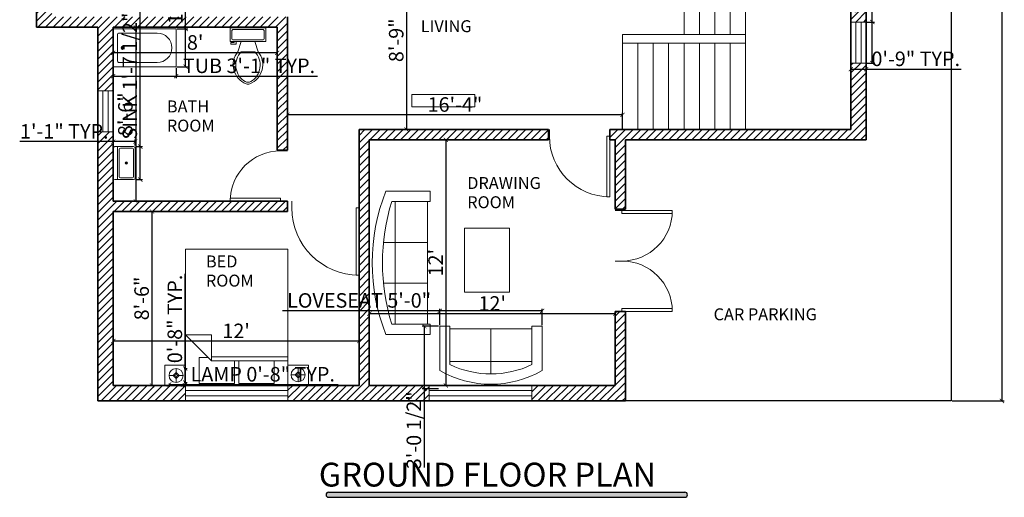
# Model space of a CAD drawing. Units: inches. Extents: x 3799 to 20199, y 1682 to 8087.
# Tile 18 of 30: x 14300 to 14876, y 2572 to 2852. Entities that reach past the tile are written whole.
import ezdxf

# ---------------------------------------------------------------- set-up
doc = ezdxf.new("R2010")
doc.units = ezdxf.units.IN
for name, color, linetype, lineweight in [('A-ANNO-DIMS', 2, 'Continuous', 18), ('A-ANNO-TITL', 7, 'Continuous', 25), ('A-AREA-IDEN', 7, 'Continuous', 18), ('A-DOOR', 3, 'Continuous', 18), ('A-FLOR-FIXT', 9, 'Continuous', 18), ('A-FLOR-STRS', 41, 'Continuous', 18), ('A-FURN', 8, 'Continuous', 18), ('A-GLAZ', 152, 'Continuous', 18), ('A-WALL', 7, 'Continuous', 35), ('A-WALL-PATT', 252, 'Continuous', 13), ('C-PROP', 7, 'Continuous', 25)]:
    doc.layers.add(name, color=color, linetype=linetype, lineweight=lineweight)
doc.styles.get("Standard").update_dxf_attribs({"font": 'arial.ttf'})
doc.dimstyles.new('ISO-25', dxfattribs={"dimtxt": 8.5, "dimasz": 2.5, "dimexe": 1.25, "dimexo": 0.625, "dimtad": 1, "dimdec": 0, "dimlunit": 3, "dimtxsty": 'Standard', "dimblk": 'ARCHTICK', "dimcen": 2.5, "dimadec": 0, "dimazin": 0, "dimtfac": 1, "dimtdec": 0, "dimtmove": 0, "dimatfit": 3, "dimfxl": 1, "dimarcsym": 0})

# ---------------------------------------------------------------- blocks, each defined once
blk = doc.blocks.new('Bed - Queen')
for p, q in [((0, -80.00003), (0, 0)), ((0, 0), (59.99999, 0)), ((59.99999, 0), (59.99999, -80.00003)), ((7.99999, -1.2), (28.79998, -1.2)), ((7.99999, -14.4), (7.99999, -1.2)), ((28.79998, -1.2), (28.79998, -14.4)), ((31.19999, -1.2), (51.99999, -1.2)), ((31.19999, -14.4), (31.19999, -1.2)), ((51.99999, -1.2), (51.99999, -16.4)), ((0, -14.4), (44.8, -14.4)), ((44.8, -16.8), (0, -16.8)), ((59.99999, -29.6), (44.8, -14.4)), ((44.8, -14.4), (44.8, -29.6)), ((51.99999, -16.4), (46.79936, -16.4)), ((44.8, -29.6), (59.99999, -29.6)), ((59.99999, -80.00003), (0, -80.00003))]:
    blk.add_line(p, q)
blk = doc.blocks.new('*U7')
for p, q in [((0, 0), (0, -100)), ((750, 0), (750, -100))]:
    blk.add_line(p, q)
blk.add_lwpolyline([(0, 0), (0, 750), (43.75, 750), (43.75, 0)], close=True)
blk.add_arc((0, 0), 750, 0, 90)
blk = doc.blocks.new('*U11')
for p, q in [((-900, 0), (-900, 100)), ((0, 0), (0, 100))]:
    blk.add_line(p, q)
blk.add_lwpolyline([(0, 0), (0, -900), (-43.75, -900), (-43.75, 0)], close=True)
blk.add_arc((0, 0), 900, 180, 270)
blk = doc.blocks.new('*U95')
for p, q in [((-1000, 0), (-1000, 100)), ((0, 0), (0, 100))]:
    blk.add_line(p, q)
blk.add_lwpolyline([(0, 0), (0, -1000), (-43.75, -1000), (-43.75, 0)], close=True)
blk.add_arc((0, 0), 1000, 180, 270)
blk = doc.blocks.new('Sofa - Roundback 7 ft.')
for p, q in [((-36.000027, -34), (-36.000027, -11.4696)), ((-12.00002, -32.4421), (-12.00003, -6.5971)), ((11.99997, -32.4421), (11.99998, -6.5971)), ((35.99998, -34), (35.99998, -11.4696)), ((-35.999844, -13.3819), (35.9998, -13.3819)), ((-36.000027, -32.4421), (35.99998, -32.4421))]:
    blk.add_line(p, q)
for points in [[(-36.000027, -34), (-42.000027, -34), (-42.000027, -8)], [(41.99998, -8), (41.99998, -34), (35.99998, -34)]]:
    blk.add_lwpolyline(points)
for centre, radius, start, end in [((0, -114.25), 114.25, 68.43141, 111.5686), ((-0.00001, -127.1968), 121.1968, 72.72033, 107.2797)]:
    blk.add_arc(centre, radius, start, end)
blk = doc.blocks.new('Sofa - Roundback Loveseat 5 ft.')
for p, q in [((-24, -33.99998), (-24, -11.46958)), ((0, -32.44198), (0, -5.99998)), ((24.00004, -33.99998), (24.00004, -11.46958)), ((-23.9998, -13.38178), (23.99986, -13.38178)), ((-24, -32.44198), (24.00004, -32.44198))]:
    blk.add_line(p, q)
for points in [[(-24, -33.99998), (-30, -33.99998), (-30, -7.99998)], [(30.00004, -7.99998), (30.00004, -33.99998), (24.00004, -33.99998)]]:
    blk.add_lwpolyline(points)
for centre, radius, start, end in [((0, -60.24998), 60.24998, 60.13715, 119.8628), ((0, -61.38438), 55.38444, 64.32083, 115.6792)]:
    blk.add_arc(centre, radius, start, end)
blk = doc.blocks.new('Lamp - Table')
for p, q in [((-1, 0), (-7, 0)), ((0, 3), (-3, 0)), ((-3, 0), (0, -3)), ((0, 7), (0, 1)), ((3, 0), (0, 3)), ((0, -3), (3, 0)), ((1, 0), (7, 0)), ((0, -1), (0, -7))]:
    blk.add_line(p, q)
for radius in [7, 1]:
    blk.add_circle((0, 0), radius)
blk = doc.blocks.new('Toilet - top')
for p, q in [((9.5, -6), (9.5, -2)), ((-10, -8.5), (-8, -8.5)), ((-10, -9.5), (-10, -8.5)), ((-7, -9.5), (-10, -9.5)), ((-8, -8.5), (-8, -8)), ((-7, -8), (-7, -9.5)), ((-4, -8), (-6, -14)), ((4, -8), (6, -14)), ((4, -14), (-4, -14))]:
    blk.add_line(p, q)
blk.add_lwpolyline([(10.5, -8), (10.5, 0), (-10.5, 0), (-10.5, -8)], close=True)
for points in [[(-9.5, -2), (-9.5, -6)], [(8.5, -1), (-8.5, -1)], [(-8.5, -7), (8.5, -7)]]:
    blk.add_lwpolyline(points)
for centre, radius, start, end in [((-8.62, -1.88), 0.884, 81.8699, 188.1301), ((8.62, -1.88), 0.884, 351.8699, 98.1301), ((-8.62, -6.12), 0.884, 171.8699, 278.1301), ((8.62, -6.12), 0.884, 261.8699, 8.1301), ((3.52, -21.58), 12.17, 141.46911, 247.97143), ((4.2, -21.82), 11.33, 136.36773, 238.94682), ((-3.52, -21.58), 12.17, 292.02843, 38.53071), ((-4.2, -21.82), 11.33, 301.05301, 43.63209), ((0, -27.88), 4, 245.73182, 294.26817), ((0, -29), 4, 254.86053, 285.13947)]:
    blk.add_arc(centre, radius, start, end)
blk = doc.blocks.new('Bath Tub - 26 x 60 in.')
for p, q in [((8, -18), (10, -18)), ((9, -17), (9, -19))]:
    blk.add_line(p, q)
blk.add_lwpolyline([(0, -36), (0, 0), (60, 0), (60, -36)], close=True)
for points in [[(4, -30), (4, -6)], [(6, -4), (42, -4)], [(42, -32), (6, -32)]]:
    blk.add_lwpolyline(points)
for radius in [1.5, 1]:
    blk.add_circle((9, -18), radius)
for centre, radius, start, end in [((5.75, -5.75), 1.77, 81.8699, 188.1301), ((42, -18), 14, 270, 90), ((5.75, -30.25), 1.77, 171.8699, 278.1301)]:
    blk.add_arc(centre, radius, start, end)
blk = doc.blocks.new('Sink-single - 30 in top')
blk.add_line((-15, -3.999996), (15, -3.999996))
for points in [[(-13.5, 0), (13.5, 0)], [(-15, -18.499996), (-15, -1.5)], [(-13.5, -17.499996), (-13.5, -6.499996)], [(-12.5, -5.499996), (12.5, -5.499996)], [(13.5, -6.499996), (13.5, -17.499996)], [(15, -1.5), (15, -18.499996)], [(13.5, -19.999996), (-13.5, -19.999996)], [(12.5, -18.499996), (-12.5, -18.499996)]]:
    blk.add_lwpolyline(points)
for radius in [1, 0.5]:
    blk.add_circle((0, -11.999996), radius)
for centre, radius, start, end in [((-13.5, -1.5), 1.5, 90, 180), ((-12.5, -6.499996), 1, 90, 180), ((12.5, -6.499996), 1, 0, 90), ((13.5, -1.5), 1.5, 0, 90), ((-12.5, -17.499996), 1, 180, 270), ((12.5, -17.499996), 1, 270, 0), ((-13.5, -18.499996), 1.5, 180, 270), ((13.5, -18.499996), 1.5, 270, 0)]:
    blk.add_arc(centre, radius, start, end)
blk = doc.blocks.new('_ArchTick')
at = {"color": 0, "linetype": 'ByBlock', "const_width": 0.15}
blk.add_lwpolyline([(-0.5, -0.5), (0.5, 0.5)], dxfattribs=at)
blk = doc.blocks.new('*D105')
at = {"layer": 'A-ANNO-DIMS', "color": 0, "lineweight": -2, "transparency": 16777216}
for p, q in [((14355.09, 2847.09), (14368.91, 2847.09)), ((14367.66, 2847.09), (14367.66, 2745.09)), ((14355.09, 2745.09), (14368.91, 2745.09))]:
    blk.add_line(p, q, dxfattribs=at)
at = {"layer": 'Defpoints', "color": 0, "transparency": 16777216}
for p in [(14354.46, 2847.09), (14354.46, 2745.09), (14367.66, 2745.09)]:
    blk.add_point(p, dxfattribs=at)
at = {"layer": 'A-ANNO-DIMS', "color": 0, "lineweight": -2, "transparency": 16777216, "xscale": 2.5, "yscale": 2.5, "zscale": 2.5}
for p, rotation in [((14367.66, 2847.09), 90), ((14367.66, 2745.09), 270)]:
    blk.add_blockref('_ArchTick', p, dxfattribs=dict(at, rotation=rotation))
at = {"layer": 'A-ANNO-DIMS', "color": 0, "transparency": 16777216, "insert": (14362.7, 2796.09), "char_height": 8.5, "attachment_point": 5, "rotation": 90}
blk.add_mtext('8\'-6"', dxfattribs=at)
blk = doc.blocks.new('*D106')
at = {"layer": 'A-ANNO-DIMS', "color": 0, "lineweight": -2, "transparency": 16777216}
for p, q in [((14354.46, 2846.47), (14354.46, 2830.85)), ((14450.46, 2846.47), (14450.46, 2830.85)), ((14450.46, 2832.1), (14354.46, 2832.1))]:
    blk.add_line(p, q, dxfattribs=at)
at = {"layer": 'Defpoints', "color": 0, "transparency": 16777216}
for p in [(14354.46, 2847.09), (14450.46, 2847.09), (14354.46, 2832.1)]:
    blk.add_point(p, dxfattribs=at)
at = {"layer": 'A-ANNO-DIMS', "color": 0, "lineweight": -2, "transparency": 16777216, "xscale": 2.5, "yscale": 2.5, "zscale": 2.5, "rotation": 180}
blk.add_blockref('_ArchTick', (14354.46, 2832.1), dxfattribs=at)
at = {"layer": 'A-ANNO-DIMS', "color": 0, "lineweight": -2, "transparency": 16777216, "xscale": 2.5, "yscale": 2.5, "zscale": 2.5}
blk.add_blockref('_ArchTick', (14450.46, 2832.1), dxfattribs=at)
at = {"layer": 'A-ANNO-DIMS', "color": 0, "transparency": 16777216, "insert": (14402.46, 2837.06), "char_height": 8.5, "attachment_point": 5}
blk.add_mtext("8'", dxfattribs=at)
blk = doc.blocks.new('*D107')
at = {"layer": 'A-ANNO-DIMS', "color": 0, "lineweight": -2, "transparency": 16777216}
for p, q in [((14354.46, 2637.72), (14354.46, 2664.35)), ((14498.46, 2637.72), (14498.46, 2664.35)), ((14498.46, 2663.1), (14354.46, 2663.1))]:
    blk.add_line(p, q, dxfattribs=at)
at = {"layer": 'Defpoints', "color": 0, "transparency": 16777216}
for p in [(14354.46, 2663.1), (14354.46, 2637.09), (14498.46, 2637.09)]:
    blk.add_point(p, dxfattribs=at)
at = {"layer": 'A-ANNO-DIMS', "color": 0, "lineweight": -2, "transparency": 16777216, "xscale": 2.5, "yscale": 2.5, "zscale": 2.5, "rotation": 180}
blk.add_blockref('_ArchTick', (14354.46, 2663.1), dxfattribs=at)
at = {"layer": 'A-ANNO-DIMS', "color": 0, "lineweight": -2, "transparency": 16777216, "xscale": 2.5, "yscale": 2.5, "zscale": 2.5}
blk.add_blockref('_ArchTick', (14498.46, 2663.1), dxfattribs=at)
at = {"layer": 'A-ANNO-DIMS', "color": 0, "transparency": 16777216, "insert": (14426.46, 2667.99), "char_height": 8.5, "attachment_point": 5}
blk.add_mtext("12'", dxfattribs=at)
blk = doc.blocks.new('*D108')
at = {"layer": 'A-ANNO-DIMS', "color": 0, "lineweight": -2, "transparency": 16777216}
for p, q in [((14355.09, 2739.09), (14378.43, 2739.09)), ((14377.18, 2739.09), (14377.18, 2637.09)), ((14355.09, 2637.09), (14378.43, 2637.09))]:
    blk.add_line(p, q, dxfattribs=at)
at = {"layer": 'Defpoints', "color": 0, "transparency": 16777216}
for p in [(14354.46, 2739.09), (14354.46, 2637.09), (14377.18, 2637.09)]:
    blk.add_point(p, dxfattribs=at)
at = {"layer": 'A-ANNO-DIMS', "color": 0, "lineweight": -2, "transparency": 16777216, "xscale": 2.5, "yscale": 2.5, "zscale": 2.5}
for p, rotation in [((14377.18, 2739.09), 90), ((14377.18, 2637.09), 270)]:
    blk.add_blockref('_ArchTick', p, dxfattribs=dict(at, rotation=rotation))
at = {"layer": 'A-ANNO-DIMS', "color": 0, "transparency": 16777216, "insert": (14372.21, 2688.09), "char_height": 8.5, "attachment_point": 5, "rotation": 90}
blk.add_mtext('8\'-6"', dxfattribs=at)
blk = doc.blocks.new('*D109')
at = {"layer": 'A-ANNO-DIMS', "color": 0, "lineweight": -2, "transparency": 16777216}
for p, q in [((14505.09, 2781.09), (14550.53, 2781.09)), ((14549.28, 2781.09), (14549.28, 2637.09)), ((14505.09, 2637.09), (14550.53, 2637.09))]:
    blk.add_line(p, q, dxfattribs=at)
at = {"layer": 'Defpoints', "color": 0, "transparency": 16777216}
for p in [(14504.46, 2781.09), (14504.46, 2637.09), (14549.28, 2637.09)]:
    blk.add_point(p, dxfattribs=at)
at = {"layer": 'A-ANNO-DIMS', "color": 0, "lineweight": -2, "transparency": 16777216, "xscale": 2.5, "yscale": 2.5, "zscale": 2.5}
for p, rotation in [((14549.28, 2781.09), 90), ((14549.28, 2637.09), 270)]:
    blk.add_blockref('_ArchTick', p, dxfattribs=dict(at, rotation=rotation))
at = {"layer": 'A-ANNO-DIMS', "color": 0, "transparency": 16777216, "insert": (14544.39, 2709.09), "char_height": 8.5, "attachment_point": 5, "rotation": 90}
blk.add_mtext("12'", dxfattribs=at)
blk = doc.blocks.new('*D110')
at = {"layer": 'A-ANNO-DIMS', "color": 0, "lineweight": -2, "transparency": 16777216}
for p, q in [((14504.46, 2637.72), (14504.46, 2680.43)), ((14648.46, 2679.18), (14504.46, 2679.18)), ((14648.46, 2637.72), (14648.46, 2680.43))]:
    blk.add_line(p, q, dxfattribs=at)
at = {"layer": 'Defpoints', "color": 0, "transparency": 16777216}
for p in [(14504.46, 2679.18), (14504.46, 2637.09), (14648.46, 2637.09)]:
    blk.add_point(p, dxfattribs=at)
at = {"layer": 'A-ANNO-DIMS', "color": 0, "lineweight": -2, "transparency": 16777216, "xscale": 2.5, "yscale": 2.5, "zscale": 2.5, "rotation": 180}
blk.add_blockref('_ArchTick', (14504.46, 2679.18), dxfattribs=at)
at = {"layer": 'A-ANNO-DIMS', "color": 0, "lineweight": -2, "transparency": 16777216, "xscale": 2.5, "yscale": 2.5, "zscale": 2.5}
blk.add_blockref('_ArchTick', (14648.46, 2679.18), dxfattribs=at)
at = {"layer": 'A-ANNO-DIMS', "color": 0, "transparency": 16777216, "insert": (14576.46, 2684.07), "char_height": 8.5, "attachment_point": 5}
blk.add_mtext("12'", dxfattribs=at)
blk = doc.blocks.new('*D111')
at = {"layer": 'A-ANNO-DIMS', "color": 0, "lineweight": -2, "transparency": 16777216}
for p, q in [((14456.46, 2787.72), (14456.46, 2796.97)), ((14652.78, 2787.72), (14652.78, 2796.97)), ((14652.78, 2795.72), (14456.46, 2795.72))]:
    blk.add_line(p, q, dxfattribs=at)
at = {"layer": 'Defpoints', "color": 0, "transparency": 16777216}
for p in [(14456.46, 2795.72), (14456.46, 2787.09), (14652.78, 2787.09)]:
    blk.add_point(p, dxfattribs=at)
at = {"layer": 'A-ANNO-DIMS', "color": 0, "lineweight": -2, "transparency": 16777216, "xscale": 2.5, "yscale": 2.5, "zscale": 2.5, "rotation": 180}
blk.add_blockref('_ArchTick', (14456.46, 2795.72), dxfattribs=at)
at = {"layer": 'A-ANNO-DIMS', "color": 0, "lineweight": -2, "transparency": 16777216, "xscale": 2.5, "yscale": 2.5, "zscale": 2.5}
blk.add_blockref('_ArchTick', (14652.78, 2795.72), dxfattribs=at)
at = {"layer": 'A-ANNO-DIMS', "color": 0, "transparency": 16777216, "insert": (14554.62, 2800.68), "char_height": 8.5, "attachment_point": 5}
blk.add_mtext('16\'-4"', dxfattribs=at)
blk = doc.blocks.new('*D112')
at = {"layer": 'A-ANNO-DIMS', "color": 0, "lineweight": -2, "transparency": 16777216}
for p, q in [((14538.58, 2891.79), (14525.03, 2891.79)), ((14526.28, 2891.79), (14526.28, 2787.09)), ((14538.58, 2787.09), (14525.03, 2787.09))]:
    blk.add_line(p, q, dxfattribs=at)
at = {"layer": 'Defpoints', "color": 0, "transparency": 16777216}
for p in [(14539.2, 2891.79), (14526.28, 2787.09), (14539.2, 2787.09)]:
    blk.add_point(p, dxfattribs=at)
at = {"layer": 'A-ANNO-DIMS', "color": 0, "lineweight": -2, "transparency": 16777216, "xscale": 2.5, "yscale": 2.5, "zscale": 2.5}
for p, rotation in [((14526.28, 2891.79), 90), ((14526.28, 2787.09), 270)]:
    blk.add_blockref('_ArchTick', p, dxfattribs=dict(at, rotation=rotation))
at = {"layer": 'A-ANNO-DIMS', "color": 0, "transparency": 16777216, "insert": (14521.32, 2839.44), "char_height": 8.5, "attachment_point": 5, "rotation": 90}
blk.add_mtext('8\'-9"', dxfattribs=at)
blk = doc.blocks.new('*D121')
at = {"layer": 'A-ANNO-DIMS', "color": 0, "lineweight": -2, "transparency": 16777216}
for p, q in [((14845.83, 3155.79), (14876.24, 3155.79)), ((14874.99, 3155.79), (14874.99, 2628.09)), ((14845.83, 2628.09), (14876.24, 2628.09))]:
    blk.add_line(p, q, dxfattribs=at)
at = {"layer": 'Defpoints', "color": 0, "transparency": 16777216}
for p in [(14845.2, 3155.79), (14845.2, 2628.09), (14874.99, 2628.09)]:
    blk.add_point(p, dxfattribs=at)
at = {"layer": 'A-ANNO-DIMS', "color": 0, "lineweight": -2, "transparency": 16777216, "xscale": 2.5, "yscale": 2.5, "zscale": 2.5}
for p, rotation in [((14874.99, 3155.79), 90), ((14874.99, 2628.09), 270)]:
    blk.add_blockref('_ArchTick', p, dxfattribs=dict(at, rotation=rotation))
at = {"layer": 'A-ANNO-DIMS', "color": 0, "transparency": 16777216, "insert": (14870.11, 2891.94), "char_height": 8.5, "attachment_point": 5, "rotation": 90}
blk.add_mtext("44'", dxfattribs=at)
blk = doc.blocks.new('WIN-24IN-9IN-FRAME')
for p, q in [((0, 24), (9, 24)), ((3, 0), (3, 24)), ((6, 0), (6, 24)), ((0, 0), (9, 0))]:
    blk.add_line(p, q)
blk = doc.blocks.new('WIN-60IN-9IN-FRAME')
for p, q in [((0, 9), (0, 0)), ((60, 6), (0, 6)), ((60, 9), (60, 0)), ((60, 3), (0, 3))]:
    blk.add_line(p, q)
blk = doc.blocks.new('*D242')
at = {"layer": 'A-ANNO-DIMS', "color": 0, "lineweight": -2, "transparency": 16777216}
for p, q in [((14799.06, 2850.1), (14799.06, 2961.41)), ((14796.09, 2850.1), (14800.31, 2850.1)), ((14799.06, 2826.1), (14799.06, 2850.1)), ((14796.09, 2826.1), (14800.31, 2826.1))]:
    blk.add_line(p, q, dxfattribs=at)
at = {"layer": 'Defpoints', "color": 0, "transparency": 16777216}
for p in [(14795.46, 2850.1), (14799.06, 2850.1), (14795.46, 2826.1)]:
    blk.add_point(p, dxfattribs=at)
at = {"layer": 'A-ANNO-DIMS', "color": 0, "lineweight": -2, "transparency": 16777216, "xscale": 2.5, "yscale": 2.5, "zscale": 2.5}
for p, rotation in [((14799.06, 2850.1), 90), ((14799.06, 2826.1), 270)]:
    blk.add_blockref('_ArchTick', p, dxfattribs=dict(at, rotation=rotation))
at = {"layer": 'A-ANNO-DIMS', "color": 0, "transparency": 16777216, "insert": (14794.04, 2907), "char_height": 8.5, "attachment_point": 5, "rotation": 90}
blk.add_mtext('WINDOW 2\'-0" TYP.', dxfattribs=at)
blk = doc.blocks.new('*D243')
at = {"layer": 'A-ANNO-DIMS', "color": 0, "lineweight": -2, "transparency": 16777216}
for p, q in [((14786.46, 2825.47), (14786.46, 2821.25)), ((14786.46, 2822.5), (14795.46, 2822.5)), ((14795.46, 2825.47), (14795.46, 2821.25)), ((14795.46, 2822.5), (14851.03, 2822.5))]:
    blk.add_line(p, q, dxfattribs=at)
at = {"layer": 'Defpoints', "color": 0, "transparency": 16777216}
for p in [(14786.46, 2826.1), (14795.46, 2826.1), (14795.46, 2822.5)]:
    blk.add_point(p, dxfattribs=at)
at = {"layer": 'A-ANNO-DIMS', "color": 0, "lineweight": -2, "transparency": 16777216, "xscale": 2.5, "yscale": 2.5, "zscale": 2.5, "rotation": 180}
blk.add_blockref('_ArchTick', (14786.46, 2822.5), dxfattribs=at)
at = {"layer": 'A-ANNO-DIMS', "color": 0, "lineweight": -2, "transparency": 16777216, "xscale": 2.5, "yscale": 2.5, "zscale": 2.5}
blk.add_blockref('_ArchTick', (14795.46, 2822.5), dxfattribs=at)
at = {"layer": 'A-ANNO-DIMS', "color": 0, "transparency": 16777216, "insert": (14824.5, 2827.46), "char_height": 8.5, "attachment_point": 5}
blk.add_mtext('0\'-9" TYP.', dxfattribs=at)
blk = doc.blocks.new('*D248')
at = {"layer": 'A-ANNO-DIMS', "color": 0, "lineweight": -2, "transparency": 16777216}
for p, q in [((14387.18, 2638.22), (14387.18, 2636.37)), ((14387.18, 2637.62), (14395.38, 2637.62)), ((14395.38, 2638.22), (14395.38, 2636.37)), ((14395.38, 2637.62), (14486.2, 2637.62))]:
    blk.add_line(p, q, dxfattribs=at)
at = {"layer": 'Defpoints', "color": 0, "transparency": 16777216}
for p in [(14387.18, 2638.85), (14395.38, 2638.85), (14395.38, 2637.62)]:
    blk.add_point(p, dxfattribs=at)
at = {"layer": 'A-ANNO-DIMS', "color": 0, "lineweight": -2, "transparency": 16777216, "xscale": 2.5, "yscale": 2.5, "zscale": 2.5, "rotation": 180}
blk.add_blockref('_ArchTick', (14387.18, 2637.62), dxfattribs=at)
at = {"layer": 'A-ANNO-DIMS', "color": 0, "lineweight": -2, "transparency": 16777216, "xscale": 2.5, "yscale": 2.5, "zscale": 2.5}
blk.add_blockref('_ArchTick', (14395.38, 2637.62), dxfattribs=at)
at = {"layer": 'A-ANNO-DIMS', "color": 0, "transparency": 16777216, "insert": (14442.04, 2642.58), "char_height": 8.5, "attachment_point": 5}
blk.add_mtext('LAMP 0\'-8" TYP.', dxfattribs=at)
blk = doc.blocks.new('*D249')
at = {"layer": 'A-ANNO-DIMS', "color": 0, "lineweight": -2, "transparency": 16777216}
for p, q in [((14396.62, 2647.05), (14396.62, 2702.62)), ((14396.01, 2647.05), (14397.87, 2647.05)), ((14396.62, 2638.85), (14396.62, 2647.05)), ((14396.01, 2638.85), (14397.87, 2638.85))]:
    blk.add_line(p, q, dxfattribs=at)
at = {"layer": 'Defpoints', "color": 0, "transparency": 16777216}
for p in [(14395.38, 2647.05), (14396.62, 2647.05), (14395.38, 2638.85)]:
    blk.add_point(p, dxfattribs=at)
at = {"layer": 'A-ANNO-DIMS', "color": 0, "lineweight": -2, "transparency": 16777216, "xscale": 2.5, "yscale": 2.5, "zscale": 2.5}
for p, rotation in [((14396.62, 2647.05), 90), ((14396.62, 2638.85), 270)]:
    blk.add_blockref('_ArchTick', p, dxfattribs=dict(at, rotation=rotation))
at = {"layer": 'A-ANNO-DIMS', "color": 0, "transparency": 16777216, "insert": (14391.65, 2676.09), "char_height": 8.5, "attachment_point": 5, "rotation": 90}
blk.add_mtext('0\'-8" TYP.', dxfattribs=at)
blk = doc.blocks.new('*D276')
at = {"layer": 'A-ANNO-DIMS', "color": 0, "lineweight": -2, "transparency": 16777216}
for p, q in [((14545.69, 2672.47), (14545.69, 2682.09)), ((14605.69, 2672.47), (14605.69, 2682.09)), ((14545.69, 2680.84), (14453.72, 2680.84)), ((14605.69, 2680.84), (14545.69, 2680.84))]:
    blk.add_line(p, q, dxfattribs=at)
at = {"layer": 'Defpoints', "color": 0, "transparency": 16777216}
for p in [(14545.69, 2680.84), (14545.69, 2671.84), (14605.69, 2671.84)]:
    blk.add_point(p, dxfattribs=at)
at = {"layer": 'A-ANNO-DIMS', "color": 0, "lineweight": -2, "transparency": 16777216, "xscale": 2.5, "yscale": 2.5, "zscale": 2.5, "rotation": 180}
blk.add_blockref('_ArchTick', (14545.69, 2680.84), dxfattribs=at)
at = {"layer": 'A-ANNO-DIMS', "color": 0, "lineweight": -2, "transparency": 16777216, "xscale": 2.5, "yscale": 2.5, "zscale": 2.5}
blk.add_blockref('_ArchTick', (14605.69, 2680.84), dxfattribs=at)
at = {"layer": 'A-ANNO-DIMS', "color": 0, "transparency": 16777216, "insert": (14498.46, 2685.86), "char_height": 8.5, "attachment_point": 5}
blk.add_mtext('LOVESEAT 5\'-0"', dxfattribs=at)
blk = doc.blocks.new('*D277')
at = {"layer": 'A-ANNO-DIMS', "color": 0, "lineweight": -2, "transparency": 16777216}
for p, q in [((14545.06, 2671.84), (14535.44, 2671.84)), ((14536.69, 2671.84), (14536.69, 2635.18)), ((14545.06, 2635.18), (14535.44, 2635.18)), ((14536.69, 2635.18), (14536.69, 2589.03))]:
    blk.add_line(p, q, dxfattribs=at)
at = {"layer": 'Defpoints', "color": 0, "transparency": 16777216}
for p in [(14545.69, 2671.84), (14536.69, 2635.18), (14545.69, 2635.18)]:
    blk.add_point(p, dxfattribs=at)
at = {"layer": 'A-ANNO-DIMS', "color": 0, "lineweight": -2, "transparency": 16777216, "xscale": 2.5, "yscale": 2.5, "zscale": 2.5}
for p, rotation in [((14536.69, 2671.84), 90), ((14536.69, 2635.18), 270)]:
    blk.add_blockref('_ArchTick', p, dxfattribs=dict(at, rotation=rotation))
at = {"layer": 'A-ANNO-DIMS', "color": 0, "transparency": 16777216, "insert": (14531.66, 2610.85), "char_height": 8.5, "attachment_point": 5, "rotation": 90}
blk.add_mtext('3\'-0 1/2"', dxfattribs=at)
blk = doc.blocks.new('*D304')
at = {"layer": 'A-ANNO-DIMS', "color": 0, "lineweight": -2, "transparency": 16777216}
for p, q in [((14354.46, 2823.32), (14354.46, 2817.17)), ((14391.34, 2823.32), (14391.34, 2817.17)), ((14354.46, 2818.42), (14391.34, 2818.42)), ((14391.34, 2818.42), (14474.17, 2818.42))]:
    blk.add_line(p, q, dxfattribs=at)
at = {"layer": 'Defpoints', "color": 0, "transparency": 16777216}
for p in [(14354.46, 2823.95), (14391.34, 2823.95), (14391.34, 2818.42)]:
    blk.add_point(p, dxfattribs=at)
at = {"layer": 'A-ANNO-DIMS', "color": 0, "lineweight": -2, "transparency": 16777216, "xscale": 2.5, "yscale": 2.5, "zscale": 2.5, "rotation": 180}
blk.add_blockref('_ArchTick', (14354.46, 2818.42), dxfattribs=at)
at = {"layer": 'A-ANNO-DIMS', "color": 0, "lineweight": -2, "transparency": 16777216, "xscale": 2.5, "yscale": 2.5, "zscale": 2.5}
blk.add_blockref('_ArchTick', (14391.34, 2818.42), dxfattribs=at)
at = {"layer": 'A-ANNO-DIMS', "color": 0, "transparency": 16777216, "insert": (14434, 2823.38), "char_height": 8.5, "attachment_point": 5}
blk.add_mtext('TUB 3\'-1" TYP.', dxfattribs=at)
blk = doc.blocks.new('*D305')
at = {"layer": 'A-ANNO-DIMS', "color": 0, "lineweight": -2, "transparency": 16777216}
for p, q in [((14396.87, 2846.08), (14396.87, 2907.44)), ((14391.97, 2846.08), (14398.12, 2846.08)), ((14396.87, 2823.95), (14396.87, 2846.08)), ((14391.97, 2823.95), (14398.12, 2823.95))]:
    blk.add_line(p, q, dxfattribs=at)
at = {"layer": 'Defpoints', "color": 0, "transparency": 16777216}
for p in [(14391.34, 2846.08), (14396.87, 2846.08), (14391.34, 2823.95)]:
    blk.add_point(p, dxfattribs=at)
at = {"layer": 'A-ANNO-DIMS', "color": 0, "lineweight": -2, "transparency": 16777216, "xscale": 2.5, "yscale": 2.5, "zscale": 2.5}
for p, rotation in [((14396.87, 2846.08), 90), ((14396.87, 2823.95), 270)]:
    blk.add_blockref('_ArchTick', p, dxfattribs=dict(at, rotation=rotation))
at = {"layer": 'A-ANNO-DIMS', "color": 0, "transparency": 16777216, "insert": (14391.91, 2878.01), "char_height": 8.5, "attachment_point": 5, "rotation": 90}
blk.add_mtext('1\'-10" TYP.', dxfattribs=at)
blk = doc.blocks.new('*D320')
at = {"layer": 'A-ANNO-DIMS', "color": 0, "lineweight": -2, "transparency": 16777216}
for p, q in [((14370.29, 2777.14), (14370.29, 2883.48)), ((14368.01, 2777.14), (14371.54, 2777.14)), ((14370.29, 2757.76), (14370.29, 2777.14)), ((14368.01, 2757.76), (14371.54, 2757.76))]:
    blk.add_line(p, q, dxfattribs=at)
at = {"layer": 'Defpoints', "color": 0, "transparency": 16777216}
for p in [(14367.39, 2777.14), (14370.29, 2777.14), (14367.39, 2757.76)]:
    blk.add_point(p, dxfattribs=at)
at = {"layer": 'A-ANNO-DIMS', "color": 0, "lineweight": -2, "transparency": 16777216, "xscale": 2.5, "yscale": 2.5, "zscale": 2.5}
for p, rotation in [((14370.29, 2777.14), 90), ((14370.29, 2757.76), 270)]:
    blk.add_blockref('_ArchTick', p, dxfattribs=dict(at, rotation=rotation))
at = {"layer": 'A-ANNO-DIMS', "color": 0, "transparency": 16777216, "insert": (14365.27, 2831.56), "char_height": 8.5, "attachment_point": 5, "rotation": 90}
blk.add_mtext('SINK 1\'-7 1/2" TYP.', dxfattribs=at)
blk = doc.blocks.new('*D321')
at = {"layer": 'A-ANNO-DIMS', "color": 0, "lineweight": -2, "transparency": 16777216}
for p, q in [((14354.46, 2780.04), (14299.7, 2780.04)), ((14354.46, 2777.76), (14354.46, 2781.29)), ((14367.39, 2780.04), (14354.46, 2780.04)), ((14367.39, 2777.76), (14367.39, 2781.29))]:
    blk.add_line(p, q, dxfattribs=at)
at = {"layer": 'Defpoints', "color": 0, "transparency": 16777216}
for p in [(14354.46, 2780.04), (14354.46, 2777.14), (14367.39, 2777.14)]:
    blk.add_point(p, dxfattribs=at)
at = {"layer": 'A-ANNO-DIMS', "color": 0, "lineweight": -2, "transparency": 16777216, "xscale": 2.5, "yscale": 2.5, "zscale": 2.5, "rotation": 180}
blk.add_blockref('_ArchTick', (14354.46, 2780.04), dxfattribs=at)
at = {"layer": 'A-ANNO-DIMS', "color": 0, "lineweight": -2, "transparency": 16777216, "xscale": 2.5, "yscale": 2.5, "zscale": 2.5}
blk.add_blockref('_ArchTick', (14367.39, 2780.04), dxfattribs=at)
at = {"layer": 'A-ANNO-DIMS', "color": 0, "transparency": 16777216, "insert": (14325.83, 2784.94), "char_height": 8.5, "attachment_point": 5}
blk.add_mtext('1\'-1" TYP.', dxfattribs=at)

msp = doc.modelspace()

# ---------------------------------------------------------------- hatches: boundary and pattern name
at = {"layer": 'A-ANNO-TITL'}
h = msp.add_hatch(color=256, dxfattribs=at)
h.dxf.hatch_style = 1
h.paths.add_polyline_path([(14689.33, 2574.54), (14480.6, 2574.54, 1), (14480.6, 2571.54), (14689.33, 2571.54, 1)])
at = {"layer": 'A-WALL-PATT'}
h = msp.add_hatch(dxfattribs=at)
h.set_pattern_fill('ANSI31', color=256)
h.paths.add_polyline_path([(14318.46, 2965.3), (14318.46, 2981.76), (14420.46, 2981.76), (14420.46, 2987.76), (14318.46, 2987.76), (14318.46, 3083.76), (14369.36, 3083.76), (14369.36, 3092.76), (14309.46, 3092.76), (14309.46, 2953.3), (14318.46, 2953.3)])
h.paths.add_polyline_path([(14456.46, 3092.76), (14393.36, 3092.76), (14393.36, 3083.76), (14450.46, 3083.76), (14450.46, 2987.76), (14450.46, 2981.76), (14450.46, 2889.09), (14456.46, 2889.09), (14456.46, 2891.79), (14539.2, 2891.79), (14539.2, 2945.79), (14533.2, 2945.79), (14533.2, 2897.79), (14456.46, 2897.79), (14456.46, 3065.79), (14474.23, 3065.79), (14474.23, 3074.79), (14456.46, 3074.79)])
h.paths.add_polyline_path([(14480.23, 3119.94, -0.534305), (14576.23, 3119.94), (14576.23, 3065.79), (14582.23, 3065.79), (14582.23, 3119.79, 0.570302), (14474.23, 3119.79), (14474.23, 3065.79), (14480.23, 3065.79)])
h.paths.add_polyline_path([(14608.2, 3146.79), (14728.2, 3146.79), (14728.2, 3109.9), (14737.2, 3109.9), (14737.2, 3155.79), (14599.2, 3155.79), (14599.2, 3074.79), (14582.23, 3074.79), (14582.23, 3065.79), (14602.2, 3065.79), (14602.2, 2936.79), (14608.2, 2936.79)])
h.paths.add_polyline_path([(14737.2, 3085.9), (14728.2, 3085.9), (14728.2, 3074.79), (14638.2, 3074.79), (14638.2, 3068.79), (14728.2, 3068.79), (14728.2, 3053.38), (14737.2, 3053.38)], flags=17)
h.paths.add_polyline_path([(14737.2, 2993.38), (14728.2, 2993.38), (14728.2, 2900.79), (14599.2, 2900.79), (14599.2, 2894.79), (14737.2, 2894.79)])
h.paths.add_polyline_path([(14795.46, 2897.45), (14791.43, 2897.45), (14791.43, 2897.79), (14772.64, 2897.79), (14772.64, 2894.79), (14786.46, 2894.79), (14786.46, 2850.1), (14795.46, 2850.1)])
h.paths.add_polyline_path([(14795.46, 2826.1), (14786.46, 2826.1), (14786.46, 2787.09), (14645.38, 2787.09), (14645.38, 2781.09), (14648.46, 2781.09), (14648.46, 2740.52), (14654.46, 2740.52), (14654.46, 2781.09), (14795.46, 2781.09)])
h.paths.add_polyline_path([(14654.46, 2680.52), (14648.46, 2680.52), (14648.46, 2637.09), (14599.58, 2637.09), (14599.58, 2628.09), (14654.46, 2628.09)])
h.paths.add_polyline_path([(14539.58, 2637.09), (14504.46, 2637.09), (14504.46, 2781.09), (14609.38, 2781.09), (14609.38, 2787.09), (14498.46, 2787.09), (14498.46, 2637.09), (14456.79, 2637.09), (14456.79, 2628.09), (14539.58, 2628.09)])
h.paths.add_polyline_path([(14396.79, 2637.09), (14384.79, 2637.09), (14354.46, 2637.09), (14354.46, 2739.09), (14456.46, 2739.09), (14456.46, 2745.09), (14354.46, 2745.09), (14354.46, 2785.72), (14345.46, 2785.72), (14345.46, 2628.09), (14396.79, 2628.09)])
h.paths.add_polyline_path([(14456.46, 2853.09), (14450.46, 2853.09), (14318.46, 2853.09), (14318.46, 2893.3), (14309.46, 2893.3), (14309.46, 2847.09), (14345.46, 2847.09), (14345.46, 2809.72), (14354.46, 2809.72), (14354.46, 2847.09), (14450.46, 2847.09), (14450.46, 2775.09), (14456.46, 2775.09)])

# ---------------------------------------------------------------- linework, layer by layer
at = {"layer": 'A-ANNO-TITL'}
for p, q in [((14480.6, 2574.54), (14689.33, 2574.54)), ((14480.6, 2571.54), (14689.33, 2571.54))]:
    msp.add_line(p, q, dxfattribs=at)
for centre, start, end in [((14480.6, 2573.04), 90, 270), ((14689.33, 2573.04), 270, 90)]:
    msp.add_arc(centre, 1.5, start, end, dxfattribs=at)
at = {"layer": 'A-FLOR-STRS'}
for p, q in [((14688.78, 2894.79), (14688.78, 2842.79)), ((14697.78, 2894.79), (14697.78, 2842.79)), ((14706.78, 2894.79), (14706.78, 2842.79)), ((14715.78, 2894.79), (14715.78, 2842.79)), ((14724.78, 2894.79), (14724.78, 2787.09)), ((14652.78, 2842.79), (14652.78, 2787.09)), ((14724.78, 2842.79), (14652.78, 2842.79)), ((14724.78, 2837.79), (14652.78, 2837.79)), ((14661.78, 2837.79), (14661.78, 2787.09)), ((14670.78, 2837.79), (14670.78, 2787.09)), ((14670.78, 2837.79), (14670.78, 2787.09)), ((14679.78, 2837.79), (14679.78, 2787.09)), ((14688.78, 2837.79), (14688.78, 2787.09)), ((14697.78, 2837.79), (14697.78, 2787.09)), ((14706.78, 2837.79), (14706.78, 2787.09)), ((14715.78, 2837.79), (14715.78, 2787.09))]:
    msp.add_line(p, q, dxfattribs=at)
at = {"layer": 'A-FURN'}
for points in [[(14529.37, 2807.66), (14566.27, 2807.66), (14566.27, 2800.34), (14529.37, 2800.34)], [(14560.19, 2729.23), (14586.57, 2729.23), (14586.57, 2691.88), (14560.19, 2691.88)], [(14396.79, 2637.09), (14384.79, 2637.09), (14384.79, 2649.09), (14396.79, 2649.09)], [(14456.79, 2637.09), (14468.79, 2637.09), (14468.79, 2649.09), (14456.79, 2649.09)]]:
    msp.add_lwpolyline(points, close=True, dxfattribs=at)
at = {"layer": 'A-WALL'}
for p, q in [((14309.46, 3092.76), (14309.46, 2847.09)), ((14795.46, 2781.09), (14795.46, 2897.45)), ((14786.46, 2787.09), (14786.46, 2894.79)), ((14456.46, 2853.09), (14456.46, 2775.09)), ((14345.46, 2847.09), (14309.46, 2847.09)), ((14345.46, 2847.09), (14345.46, 2628.09)), ((14450.46, 2847.09), (14354.46, 2847.09)), ((14354.46, 2847.09), (14354.46, 2745.09)), ((14450.46, 2847.09), (14450.46, 2775.09)), ((14498.46, 2787.09), (14498.46, 2637.09)), ((14609.38, 2787.09), (14498.46, 2787.09)), ((14609.38, 2781.09), (14609.38, 2787.09)), ((14786.46, 2787.09), (14645.38, 2787.09)), ((14645.38, 2781.09), (14645.38, 2787.09)), ((14504.46, 2781.09), (14504.46, 2637.09)), ((14609.38, 2781.09), (14504.46, 2781.09)), ((14648.46, 2781.09), (14645.38, 2781.09)), ((14648.46, 2781.09), (14648.46, 2740.52)), ((14795.46, 2781.09), (14654.46, 2781.09)), ((14654.46, 2781.09), (14654.46, 2740.52)), ((14456.46, 2775.09), (14450.46, 2775.09)), ((14456.46, 2745.09), (14354.46, 2745.09)), ((14456.46, 2745.09), (14456.46, 2739.09)), ((14648.46, 2740.52), (14654.46, 2740.52)), ((14456.46, 2739.09), (14354.46, 2739.09)), ((14354.46, 2739.09), (14354.46, 2637.09)), ((14648.46, 2680.52), (14654.46, 2680.52)), ((14648.46, 2680.52), (14648.46, 2637.09)), ((14654.46, 2680.52), (14654.46, 2628.09)), ((14498.46, 2637.09), (14354.46, 2637.09)), ((14648.46, 2637.09), (14504.46, 2637.09)), ((14654.46, 2628.09), (14345.46, 2628.09))]:
    msp.add_line(p, q, dxfattribs=at)
at = {"layer": 'C-PROP'}
for p, q in [((14845.2, 3155.79), (14845.2, 2628.09)), ((14845.2, 2628.09), (14654.46, 2628.09))]:
    msp.add_line(p, q, dxfattribs=at)

# ---------------------------------------------------------------- block references
at = {"layer": 'A-DOOR', "xscale": 0.0393700787401575, "yscale": 0.0393700787401575, "zscale": 0.0393700787401575}
for name, p in [('*U11', (14645.38, 2783.15)), ('*U95', (14498.46, 2741.15))]:
    msp.add_blockref(name, p, dxfattribs=at)
at = {"layer": 'A-DOOR', "yscale": 0.0393700787401575, "zscale": 0.0393700787401575}
for p, xscale, rotation in [((14452.53, 2745.09), 0.0393700787401575, 90), ((14652.4, 2739.58), 0.0393700787401575, 270), ((14652.4, 2680.52), -0.0393700787401575, 270)]:
    msp.add_blockref('*U7', p, dxfattribs=dict(at, xscale=xscale, rotation=rotation))
at = {"layer": 'A-FLOR-FIXT', "xscale": 0.6146362971528592, "yscale": 0.6146362971528592, "zscale": 0.6146362971528592}
msp.add_blockref('Bath Tub - 26 x 60 in.', (14354.46, 2846.08), dxfattribs=at)
at = {"layer": 'A-FLOR-FIXT'}
msp.add_blockref('Toilet - top', (14433.41, 2846.71), dxfattribs=at)
at = {"layer": 'A-FLOR-FIXT', "xscale": 0.6460358096658105, "yscale": 0.6460358096658105, "zscale": 0.6460358096658105, "rotation": 90}
msp.add_blockref('Sink-single - 30 in top', (14354.46, 2767.45), dxfattribs=at)
at = {"layer": 'A-FURN'}
for name, p, rotation in [('Sofa - Roundback 7 ft.', (14506.18, 2708.99), 90), ('Bed - Queen', (14456.79, 2637.09), 180), ('Sofa - Roundback Loveseat 5 ft.', (14575.69, 2637.84), 180)]:
    msp.add_blockref(name, p, dxfattribs=dict(at, rotation=rotation))
at = {"layer": 'A-FURN', "xscale": 0.5860159880705021, "yscale": 0.5860159880705021, "zscale": 0.5860159880705021}
for p in [(14391.28, 2642.95), (14462.74, 2643.37)]:
    msp.add_blockref('Lamp - Table', p, dxfattribs=at)
at = {"layer": 'A-GLAZ'}
for name, p in [('WIN-24IN-9IN-FRAME', (14786.46, 2826.1)), ('WIN-24IN-9IN-FRAME', (14345.46, 2785.72)), ('WIN-60IN-9IN-FRAME', (14396.79, 2628.09)), ('WIN-60IN-9IN-FRAME', (14539.58, 2628.09))]:
    msp.add_blockref(name, p, dxfattribs=at)

# ---------------------------------------------------------------- texts
at = {"layer": 'A-ANNO-TITL'}
msp.add_text('GROUND FLOOR PLAN', height=13.966, rotation=0.00194, dxfattribs=at).set_placement((14474.89, 2577.86))
at = {"layer": 'A-AREA-IDEN'}
for s, p in [('LIVING', (14534.6, 2844.19)), ('BATH', (14385.9, 2797.16)), ('ROOM', (14385.9, 2785.92)), ('DRAWING', (14561.81, 2752.26)), ('ROOM', (14561.81, 2741.01)), ('BED', (14408.77, 2706.3)), ('ROOM', (14408.77, 2695.06)), ('CAR PARKING', (14706.11, 2675.31))]:
    msp.add_text(s, height=7, rotation=0.00194, dxfattribs=at).set_placement(p)

# ---------------------------------------------------------------- dimensions: what is measured, and where the dimension line sits
at = {"layer": 'A-ANNO-DIMS'}
for base, p1, p2, angle, override, picture, middle in [((14874.99, 2628.09), (14845.2, 3155.79), (14845.2, 2628.09), 90, {"dimclrd": 0, "dimclre": 0, "dimclrt": 0}, '*D121', (14870.11, 2891.94)), ((14526.28, 2787.09), (14539.2, 2891.79), (14539.2, 2787.09), 90, {"dimclrd": 0, "dimclre": 0, "dimclrt": 0}, '*D112', (14521.32, 2839.44)), ((14377.18, 2637.09), (14354.46, 2739.09), (14354.46, 2637.09), 90, {"dimclrd": 0, "dimclre": 0, "dimclrt": 0}, '*D108', (14372.21, 2688.09)), ((14536.69, 2635.18), (14545.69, 2671.84), (14545.69, 2635.18), 270, {"dimdec": 1, "dimlfac": 1, "dimrnd": 0, "dimzin": 1, "dimdsep": 46, "dimlunit": 4, "dimfrac": 2}, '*D277', (14531.66, 2610.85))]:
    dim = msp.add_linear_dim(base=base, p1=p1, p2=p2, angle=angle, dimstyle='ISO-25', override=override, dxfattribs=at)
    dim.commit()
    dim.dimension.update_dxf_attribs({"geometry": picture, "text_midpoint": middle})
for base, p1, p2, angle, text, picture, middle in [((14799.06, 2850.1), (14795.46, 2826.1), (14795.46, 2850.1), 90, 'WINDOW <> TYP.', '*D242', (14794.04, 2907)), ((14396.87, 2846.08), (14391.34, 2823.95), (14391.34, 2846.08), 90, '<> TYP.', '*D305', (14391.91, 2878.01)), ((14370.29, 2777.14), (14367.39, 2757.76), (14367.39, 2777.14), 90, 'SINK <> TYP.', '*D320', (14365.27, 2831.56)), ((14354.46, 2780.04), (14367.39, 2777.14), (14354.46, 2777.14), 180, '<> TYP.', '*D321', (14325.83, 2784.94)), ((14396.62, 2647.05), (14395.38, 2638.85), (14395.38, 2647.05), 90, '<> TYP.', '*D249', (14391.65, 2676.09)), ((14545.69, 2680.84), (14605.69, 2671.84), (14545.69, 2671.84), 180, 'LOVESEAT <>', '*D276', (14498.46, 2685.86))]:
    dim = msp.add_linear_dim(base=base, p1=p1, p2=p2, angle=angle, text=text, dimstyle='ISO-25', override={"dimdec": 1, "dimlfac": 1, "dimrnd": 0, "dimzin": 1, "dimdsep": 46, "dimlunit": 4, "dimfrac": 2}, dxfattribs=at)
    dim.commit()
    dim.dimension.update_dxf_attribs({"geometry": picture, "text_midpoint": middle})
for base, p1, p2, picture, middle in [((14354.46, 2832.1), (14450.46, 2847.09), (14354.46, 2847.09), '*D106', (14402.46, 2837.06)), ((14456.46, 2795.72), (14652.78, 2787.09), (14456.46, 2787.09), '*D111', (14554.62, 2800.68)), ((14504.46, 2679.18), (14648.46, 2637.09), (14504.46, 2637.09), '*D110', (14576.46, 2684.07)), ((14354.46, 2663.1), (14498.46, 2637.09), (14354.46, 2637.09), '*D107', (14426.46, 2667.99))]:
    dim = msp.add_linear_dim(base=base, p1=p1, p2=p2, dimstyle='ISO-25', override={"dimclrd": 0, "dimclre": 0, "dimclrt": 0}, dxfattribs=at)
    dim.commit()
    dim.dimension.update_dxf_attribs({"geometry": picture, "text_midpoint": middle})
for base, p1, p2, text, picture, middle in [((14391.34, 2818.42), (14354.46, 2823.95), (14391.34, 2823.95), 'TUB <> TYP.', '*D304', (14434, 2823.38)), ((14795.46, 2822.5), (14786.46, 2826.1), (14795.46, 2826.1), '<> TYP.', '*D243', (14824.5, 2827.46)), ((14395.38, 2637.62), (14387.18, 2638.85), (14395.38, 2638.85), 'LAMP <> TYP.', '*D248', (14442.04, 2642.58))]:
    dim = msp.add_linear_dim(base=base, p1=p1, p2=p2, text=text, dimstyle='ISO-25', override={"dimdec": 1, "dimlfac": 1, "dimrnd": 0, "dimzin": 1, "dimdsep": 46, "dimlunit": 4, "dimfrac": 2}, dxfattribs=at)
    dim.commit()
    dim.dimension.update_dxf_attribs({"geometry": picture, "text_midpoint": middle})
for p1, p2, distance, picture, middle in [((14354.46, 2847.09), (14354.46, 2745.09), 13.2, '*D105', (14362.7, 2796.09)), ((14504.46, 2781.09), (14504.46, 2637.09), 44.81, '*D109', (14544.39, 2709.09))]:
    dim = msp.add_aligned_dim(p1=p1, p2=p2, distance=distance, dimstyle='ISO-25', override={"dimclrd": 0, "dimclre": 0, "dimclrt": 0}, dxfattribs=at)
    dim.commit()
    dim.dimension.update_dxf_attribs({"geometry": picture, "text_midpoint": middle})

doc.saveas('drawing.dxf')
